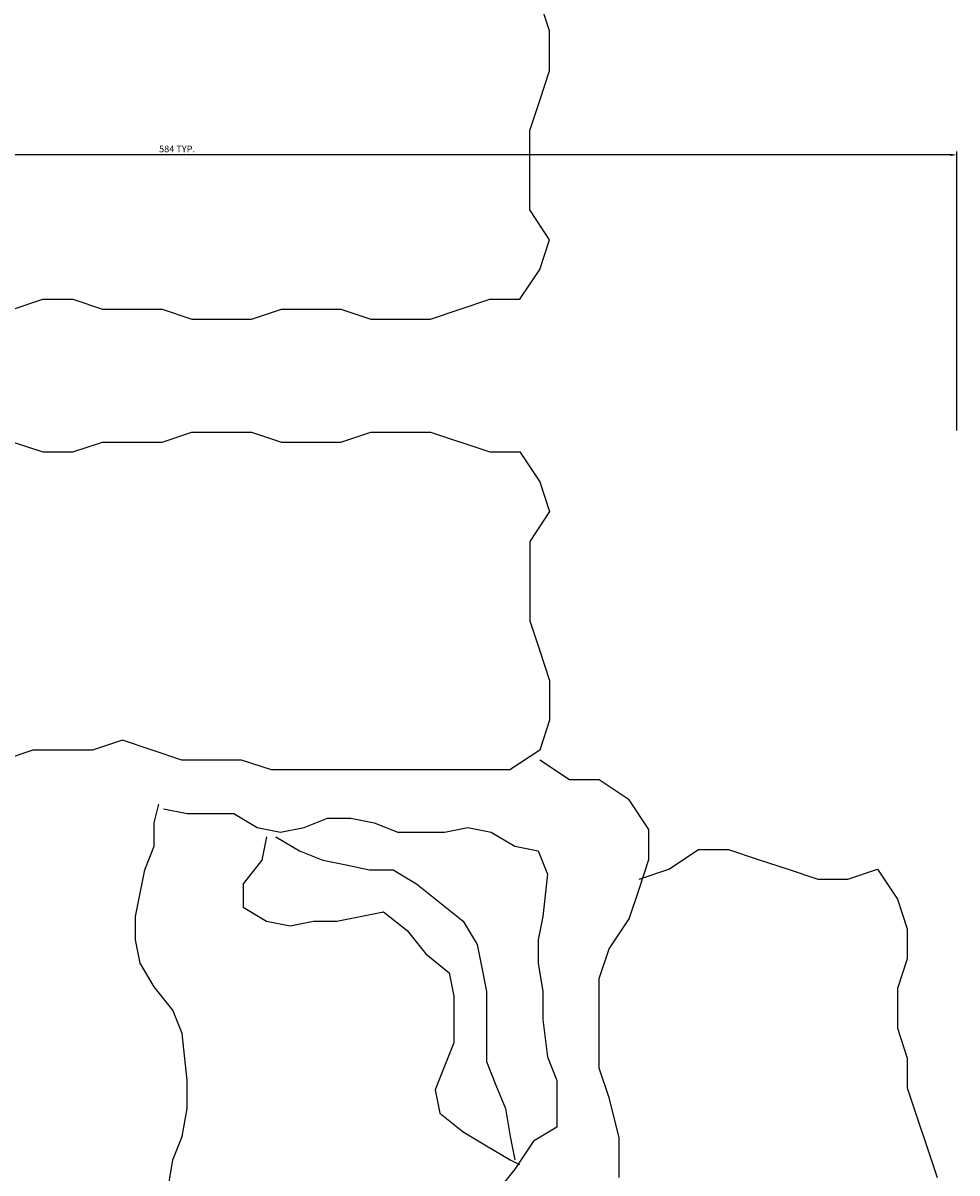
# Model space of a CAD drawing. Units: millimetres. Extents: x -857 to 54106, y -13666 to 13947.
# Tile 26 of 41: x 29011 to 29360, y 10747 to 11178. Entities that reach past the tile are written whole.
import ezdxf

# ---------------------------------------------------------------- set-up
doc = ezdxf.new("R2010")
doc.units = ezdxf.units.MM
doc.layers.add('A-ANNO-DIMS', color=2, linetype='Continuous', lineweight=18)
doc.layers.add('A-FURN', color=21, linetype='Continuous', lineweight=18)
doc.layers.add('TEFRIŞ', color=11, linetype='Continuous')
doc.styles.get("Standard").update_dxf_attribs({"font": 'arial.ttf'})
doc.dimstyles.new('ISO-25', dxfattribs={"dimtxt": 2.5, "dimasz": 2.5, "dimexe": 1.25, "dimexo": 0.625, "dimtad": 1, "dimtxsty": 'Standard', "dimcen": 2.5, "dimadec": 0, "dimazin": 0, "dimtfac": 1, "dimtmove": 0, "dimatfit": 3, "dimfxl": 1, "dimarcsym": 0})

# ---------------------------------------------------------------- blocks, each defined once
blk = doc.blocks.new('25')
at = {"layer": 'TEFRIŞ'}
for p, q in [((-1947.431, -352.718), (-1946.503, -351.558)), ((-1930.277, -351.79), (-1930.509, -353.182)), ((-1967.852, -353.796), (-1968.344, -352.319)), ((-1952.602, -352.319), (-1952.602, -354.288)), ((-1948.358, -354.11), (-1947.431, -352.718)), ((-1947.199, -353.182), (-1947.663, -352.95)), ((-1947.199, -354.342), (-1947.431, -353.182)), ((-1946.04, -353.878), (-1947.199, -353.182)), ((-1930.509, -353.182), (-1930.972, -354.342)), ((-1967.36, -355.273), (-1967.852, -353.796)), ((-1952.602, -354.288), (-1952.11, -356.258)), ((-1949.517, -354.806), (-1948.358, -354.11)), ((-1946.967, -355.733), (-1947.199, -354.342)), ((-1944.881, -354.574), (-1946.04, -353.878)), ((-1930.972, -354.342), (-1931.204, -355.733)), ((-1949.517, -357.125), (-1949.517, -354.806)), ((-1943.722, -355.501), (-1944.881, -354.574)), ((-1966.869, -356.75), (-1967.36, -355.273)), ((-1943.49, -356.661), (-1943.722, -355.501)), ((-1946.503, -356.893), (-1946.967, -355.733)), ((-1931.204, -355.733), (-1931.204, -357.125)), ((-1952.11, -356.258), (-1951.618, -357.734)), ((-1966.869, -358.227), (-1966.869, -356.75)), ((-1949.053, -358.285), (-1949.517, -357.125)), ((-1946.04, -358.053), (-1946.503, -356.893)), ((-1943.954, -357.821), (-1943.49, -356.661)), ((-1931.204, -357.125), (-1930.972, -359.445)), ((-1951.618, -357.734), (-1951.618, -362.165)), ((-1966.377, -359.704), (-1966.869, -358.227)), ((-1948.822, -360.141), (-1949.053, -358.285)), ((-1946.04, -361.532), (-1946.04, -358.053)), ((-1944.417, -358.981), (-1943.954, -357.821)), ((-1944.417, -361.301), (-1944.417, -358.981)), ((-1930.972, -359.445), (-1930.509, -360.605)), ((-1966.377, -361.673), (-1966.377, -359.704)), ((-1948.822, -361.532), (-1948.822, -360.141)), ((-1930.509, -360.605), (-1929.582, -361.764)), ((-1966.869, -363.15), (-1966.377, -361.673)), ((-1948.59, -362.924), (-1948.822, -361.532)), ((-1945.808, -362.692), (-1946.04, -361.532)), ((-1944.185, -362.46), (-1944.417, -361.301)), ((-1929.582, -361.764), (-1928.886, -362.924)), ((-1951.618, -362.165), (-1952.11, -363.642)), ((-1948.59, -364.084), (-1948.59, -362.924)), ((-1945.576, -363.852), (-1945.808, -362.692)), ((-1943.026, -363.388), (-1944.185, -362.46)), ((-1928.886, -362.924), (-1928.654, -364.084)), ((-1966.869, -364.626), (-1966.869, -363.15)), ((-1942.099, -364.548), (-1943.026, -363.388)), ((-1952.11, -363.642), (-1953.094, -365.119)), ((-1944.881, -365.012), (-1945.576, -363.852)), ((-1966.377, -366.103), (-1966.869, -364.626)), ((-1948.822, -365.244), (-1948.59, -364.084)), ((-1940.94, -365.476), (-1942.099, -364.548)), ((-1928.654, -364.084), (-1928.654, -365.244)), ((-1953.094, -365.119), (-1953.586, -366.596)), ((-1943.722, -365.94), (-1944.881, -365.012)), ((-1938.622, -365.012), (-1939.781, -365.244)), ((-1937.463, -365.012), (-1938.622, -365.012)), ((-1936.304, -364.78), (-1937.463, -365.012)), ((-1935.145, -365.012), (-1936.304, -364.78)), ((-1933.986, -365.708), (-1935.145, -365.012)), ((-1949.053, -367.332), (-1948.822, -365.244)), ((-1939.781, -365.244), (-1940.94, -365.476)), ((-1933.986, -366.868), (-1933.986, -365.708)), ((-1928.654, -365.244), (-1928.886, -366.404)), ((-1965.393, -367.58), (-1966.377, -366.103)), ((-1942.563, -366.868), (-1943.722, -365.94)), ((-1953.586, -366.596), (-1954.078, -368.072)), ((-1941.404, -367.563), (-1942.563, -366.868)), ((-1934.913, -368.027), (-1933.986, -366.868)), ((-1928.886, -366.404), (-1929.118, -367.563)), ((-1963.917, -367.088), (-1965.393, -367.58)), ((-1962.441, -367.088), (-1963.917, -367.088)), ((-1960.965, -367.58), (-1962.441, -367.088)), ((-1953.586, -367.088), (-1955.062, -367.58)), ((-1948.59, -368.491), (-1949.053, -367.332)), ((-1959.489, -368.072), (-1960.965, -367.58)), ((-1955.062, -367.58), (-1956.537, -368.565)), ((-1940.245, -367.563), (-1941.404, -367.563)), ((-1939.086, -367.795), (-1940.245, -367.563)), ((-1937.927, -368.027), (-1939.086, -367.795)), ((-1936.768, -368.491), (-1937.927, -368.027)), ((-1935.145, -369.187), (-1934.913, -368.027)), ((-1929.118, -367.563), (-1929.582, -368.723)), ((-1958.013, -368.565), (-1959.489, -368.072)), ((-1956.537, -368.565), (-1958.013, -368.565)), ((-1954.078, -368.072), (-1954.078, -369.549)), ((-1947.431, -368.723), (-1948.59, -368.491)), ((-1935.609, -369.187), (-1936.768, -368.491)), ((-1946.272, -369.419), (-1947.431, -368.723)), ((-1929.582, -368.723), (-1929.582, -369.883)), ((-1954.078, -369.549), (-1953.094, -371.026)), ((-1945.113, -369.651), (-1946.272, -369.419)), ((-1943.954, -369.419), (-1945.113, -369.651)), ((-1941.636, -369.419), (-1943.954, -369.419)), ((-1940.477, -369.883), (-1941.636, -369.419)), ((-1936.999, -369.651), (-1938.158, -370.115)), ((-1935.84, -369.419), (-1936.999, -369.651)), ((-1934.681, -369.651), (-1935.84, -369.419)), ((-1933.522, -370.347), (-1934.681, -369.651)), ((-1939.317, -370.115), (-1940.477, -369.883)), ((-1938.158, -370.115), (-1939.317, -370.115)), ((-1929.582, -369.883), (-1929.813, -370.811)), ((-1931.204, -370.347), (-1933.522, -370.347)), ((-1930.045, -370.579), (-1931.204, -370.347)), ((-1953.094, -371.026), (-1951.618, -372.011)), ((-1951.618, -372.011), (-1950.142, -372.011)), ((-1950.142, -372.011), (-1948.666, -372.995)), ((-1948.666, -373.488), (-1947.19, -372.503)), ((-1947.19, -372.503), (-1935.383, -372.503)), ((-1935.383, -372.503), (-1933.907, -372.995)), ((-1933.907, -372.995), (-1930.956, -372.995)), ((-1930.956, -372.995), (-1929.48, -373.488)), ((-1923.576, -373.488), (-1922.101, -372.995)), ((-1949.158, -374.964), (-1948.666, -373.488)), ((-1929.48, -373.488), (-1928.004, -373.98)), ((-1928.004, -373.98), (-1926.528, -373.488)), ((-1926.528, -373.488), (-1923.576, -373.488)), ((-1949.158, -376.934), (-1949.158, -374.964)), ((-1948.666, -378.41), (-1949.158, -376.934)), ((-1948.174, -379.887), (-1948.666, -378.41)), ((-1948.174, -383.826), (-1948.174, -379.887)), ((-1949.158, -385.303), (-1948.174, -383.826)), ((-1948.666, -386.779), (-1949.158, -385.303)), ((-1947.682, -388.256), (-1948.666, -386.779)), ((-1946.206, -388.256), (-1947.682, -388.256)), ((-1943.255, -389.241), (-1946.206, -388.256)), ((-1925.544, -388.256), (-1927.02, -388.749)), ((-1924.068, -388.256), (-1925.544, -388.256)), ((-1922.592, -388.749), (-1924.068, -388.256)), ((-1938.827, -388.749), (-1940.303, -389.241)), ((-1935.875, -388.749), (-1938.827, -388.749)), ((-1934.399, -389.241), (-1935.875, -388.749)), ((-1929.972, -388.749), (-1931.448, -389.241)), ((-1927.02, -388.749), (-1929.972, -388.749)), ((-1940.303, -389.241), (-1943.255, -389.241)), ((-1931.448, -389.241), (-1934.399, -389.241))]:
    blk.add_line(p, q, dxfattribs=at)
blk = doc.blocks.new('*D50')
at = {"layer": 'A-ANNO-DIMS', "color": 0, "lineweight": -2, "transparency": 16777216}
for p, q in [((28776.63, 11025.41), (28776.63, 11129.86)), ((29360.48, 11025.41), (29360.48, 11129.86)), ((29357.98, 11128.61), (28779.13, 11128.61))]:
    blk.add_line(p, q, dxfattribs=at)
at = {"layer": 'A-ANNO-DIMS', "color": 0, "transparency": 16777216}
for points in [[(28779.13, 11129.03), (28779.13, 11128.19), (28776.63, 11128.61)], [(29357.98, 11129.03), (29357.98, 11128.19), (29360.48, 11128.61)]]:
    blk.add_solid(points, dxfattribs=at)
at = {"layer": 'Defpoints', "color": 0, "transparency": 16777216}
for p in [(28776.63, 11128.61), (28776.63, 11024.79), (29360.48, 11024.79)]:
    blk.add_point(p, dxfattribs=at)
at = {"layer": 'A-ANNO-DIMS', "color": 0, "transparency": 16777216, "insert": (29068.56, 11130.51), "char_height": 2.5, "attachment_point": 5}
blk.add_mtext('584 TYP.', dxfattribs=at)

msp = doc.modelspace()

# ---------------------------------------------------------------- block references
at = {"layer": 'A-FURN', "xscale": -7.559220362162901, "yscale": 7.559220362162901, "zscale": 7.559220362162901}
msp.add_blockref('25', (14473.896, 14009.447), dxfattribs=at)
at = {"layer": 'A-FURN', "xscale": 7.559220362162901, "yscale": 7.559220362162901, "zscale": 7.559220362162901, "rotation": 180}
msp.add_blockref('25', (14473.896, 8082.429), dxfattribs=at)

# ---------------------------------------------------------------- dimensions: what is measured, and where the dimension line sits
at = {"layer": 'A-ANNO-DIMS'}
dim = msp.add_linear_dim(base=(28776.63, 11128.611), p1=(29360.482, 11024.786), p2=(28776.63, 11024.786), angle=180, text='<> TYP.', dimstyle='ISO-25', override={"dimdec": 0, "dimrnd": 0, "dimzin": 0, "dimlunit": 2}, dxfattribs=at)
dim.commit()
dim.dimension.update_dxf_attribs({"geometry": '*D50', "text_midpoint": (29068.556, 11130.512)})

doc.saveas('drawing.dxf')
